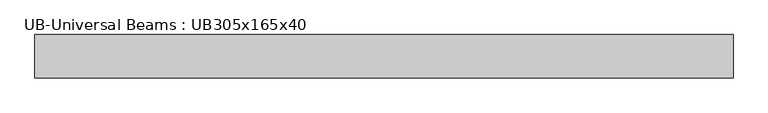
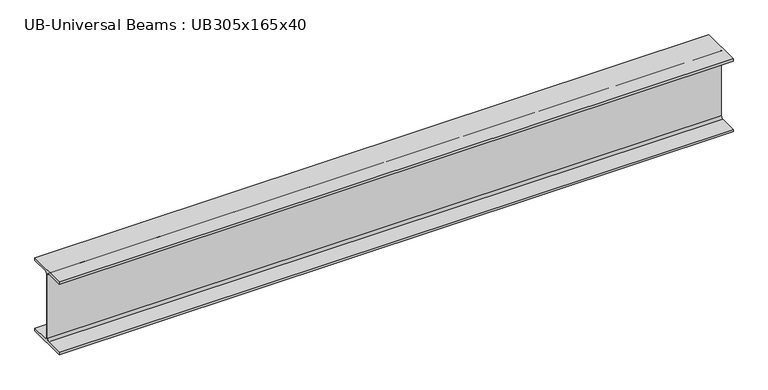
"""IFC4 building model written with IfcOpenShell, lengths in millimetres: beam geometry, UB-Universal Beams : UB305x165x40."""

from ifc_helpers import new_model, si_unit, point, frame, frame_2d, origin, place, context, project, spatial, polyline, circle_curve, trimmed, segment, composite_curve, outline, extrude, source, transform, mapped, element, save


def ub_universal_beams_ub305x165x40_60ab2ee1(model_context):
    return source(origin(), model_context, "Body", "SweptSolid", [
        extrude(outline(composite_curve([segment(polyline([(82.5, -141.5), (82.5, -151.7), (-82.5, -151.7), (-82.5, -141.5), (-11.9, -141.5)]), True, "CONTINUOUS"), segment(trimmed(circle_curve(frame_2d((-11.9, -132.6)), 8.9), [point((-11.9, -141.5))], [point((-3.0, -132.6))], True, "CARTESIAN"), True, "CONTINUOUS"), segment(polyline([(-3.0, -132.6), (-3.0, 132.6)]), True, "CONTINUOUS"), segment(trimmed(circle_curve(frame_2d((-11.9, 132.6)), 8.9), [point((-3.0, 132.6))], [point((-11.9, 141.5))], True, "CARTESIAN"), True, "CONTINUOUS"), segment(polyline([(-11.9, 141.5), (-82.5, 141.5), (-82.5, 151.7), (82.5, 151.7), (82.5, 141.5), (11.9, 141.5)]), True, "CONTINUOUS"), segment(trimmed(circle_curve(frame_2d((11.9, 132.6)), 8.9), [point((11.9, 141.5))], [point((3.0, 132.6))], True, "CARTESIAN"), True, "CONTINUOUS"), segment(polyline([(3.0, 132.6), (3.0, -132.6)]), True, "CONTINUOUS"), segment(trimmed(circle_curve(frame_2d((11.9, -132.6)), 8.9), [point((3.0, -132.6))], [point((11.9, -141.5))], True, "CARTESIAN"), True, "CONTINUOUS"), segment(polyline([(11.9, -141.5), (82.5, -141.5)]), True, "CONTINUOUS")], self_intersect=False)), frame((-1324.7, 0.0, 0.0), z_axis=(1.0, 0.0, 0.0), x_axis=(0.0, 1.0, 0.0)), (0.0, 0.0, 1.0), 2649.4),
    ])


if __name__ == "__main__":
    model = new_model("IFC4")
    model_context = context("Model", 3, world=origin())
    ifc_project = project(units=[si_unit("LENGTHUNIT", "METRE", prefix="MILLI")], contexts=[model_context])
    site = spatial("IfcSite", under=ifc_project)
    building = spatial("IfcBuilding", under=site)
    placement = place(None, origin())
    ub_universal_beams_ub305x165x40_shape = ub_universal_beams_ub305x165x40_60ab2ee1(model_context)
    element("IfcBeam", 1, ObjectType="UB-Universal Beams : UB305x165x40", at=placement, inside=building, context=model_context, shape_type="MappedRepresentation", body=[
        mapped(ub_universal_beams_ub305x165x40_shape, transform((0.0, 0.0, 0.0), x_axis=(1.0, 0.0, 0.0), y_axis=(0.0, 1.0, 0.0), z_axis=(0.0, 0.0, 1.0))),
    ])
    save(model, "model.ifc")

# Revit data of these elements
# Type "UB-Universal Beams : UB305x165x40"
#   Section Name Key = "UB305X165X40"
#   Width = 16.5 cm
#   Web Thickness = 0.6 cm
#   Web Fillet = 0.89 cm
#   Warping Constant = 164000.0 cm⁶
#   Torsional Moment of Inertia = 14.70 cm⁴
#   Section Area = 51.3 cm²
#   Plastic Modulus weak axis = 142.0 cm³
#   Plastic Modulus strong axis = 623.0 cm³
#   Nominal Weight = 40.2999 kgf/m
#   Moment of Inertia weak axis = 764.00 cm⁴
#   Moment of Inertia strong axis = 8503.00 cm⁴
#   Height = 30.34 cm
#   Flange Thickness = 1.02 cm
#   Elastic Modulus weak axis = 92.6 cm³
#   Elastic Modulus strong axis = 560.0 cm³
#   Centroid Vertical = 15.17 cm
#   Centroid Horizontal = 8.25 cm
#   Bolt Spacing = 9.0 cm
#   Length [instance default] = 1.5 m
#   Structural Material [instance default] = Metal - Steel 43-275
#   Type Comments = ""
#   Assembly Code = ""
# Element 1 (IfcBeam, "UB-Universal Beams : UB305x165x40")
#   Materials on its faces: "Metal - Steel 43-275"
# Materials
#   "Metal - Steel 43-275": class "Metal", colour RGB 247 247 247, transparency 0, Cost = 0
